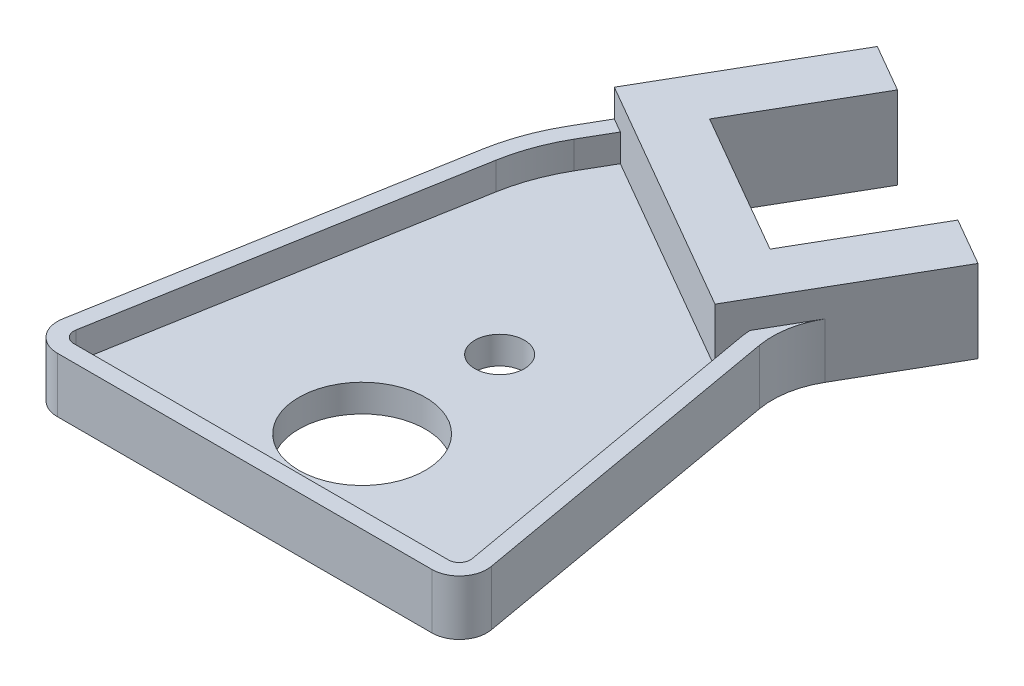
ISO-10303-21;
HEADER;
FILE_DESCRIPTION(('STEP AP214'),'2;1');
FILE_NAME('part.step','',(''),(''),'','','');
FILE_SCHEMA(('AUTOMOTIVE_DESIGN { 1 0 10303 214 1 1 1 1 }'));
ENDSEC;
DATA;
#1=APPLICATION_CONTEXT('core data for automotive mechanical design processes');
#2=APPLICATION_PROTOCOL_DEFINITION('international standard','automotive_design',2000,#1);
#3=PRODUCT_CONTEXT('',#1,'mechanical');
#4=PRODUCT('Part','Part','',(#3));
#5=PRODUCT_RELATED_PRODUCT_CATEGORY('part','',(#4));
#6=PRODUCT_DEFINITION_FORMATION('','',#4);
#7=PRODUCT_DEFINITION_CONTEXT('part definition',#1,'design');
#8=PRODUCT_DEFINITION('design','',#6,#7);
#9=PRODUCT_DEFINITION_SHAPE('','',#8);
#10=(LENGTH_UNIT() NAMED_UNIT(*) SI_UNIT(.MILLI.,.METRE.));
#11=(NAMED_UNIT(*) PLANE_ANGLE_UNIT() SI_UNIT($,.RADIAN.));
#12=(NAMED_UNIT(*) SI_UNIT($,.STERADIAN.) SOLID_ANGLE_UNIT());
#13=UNCERTAINTY_MEASURE_WITH_UNIT(LENGTH_MEASURE(1.E-05),#10,'distance_accuracy_value','');
#14=(GEOMETRIC_REPRESENTATION_CONTEXT(3) GLOBAL_UNCERTAINTY_ASSIGNED_CONTEXT((#13)) GLOBAL_UNIT_ASSIGNED_CONTEXT((#10,
#11,#12)) REPRESENTATION_CONTEXT('',''));
#15=CARTESIAN_POINT('',(0.,0.,0.));
#16=DIRECTION('',(0.,0.,1.));
#17=DIRECTION('',(1.,0.,0.));
#18=AXIS2_PLACEMENT_3D('',#15,#16,#17);
#19=CARTESIAN_POINT('',(5.58841015037912,10.,-64.6794103139903));
#20=DIRECTION('',(0.,-1.,0.));
#21=DIRECTION('',(0.,0.,-1.));
#22=AXIS2_PLACEMENT_3D('',#19,#20,#21);
#23=CYLINDRICAL_SURFACE('',#22,32.);
#24=CARTESIAN_POINT('',(5.58841015037912,5.,-64.6794103139903));
#25=DIRECTION('',(0.,1.,0.));
#26=DIRECTION('',(0.,0.,1.));
#27=AXIS2_PLACEMENT_3D('',#24,#25,#26);
#28=CIRCLE('',#27,32.);
#29=CARTESIAN_POINT('',(-22.1244027707229,5.,-80.6794103139904));
#30=VERTEX_POINT('',#29);
#31=CARTESIAN_POINT('',(-25.9254379460116,5.,-70.2361519993319));
#32=VERTEX_POINT('',#31);
#33=EDGE_CURVE('E290',#30,#32,#28,.T.);
#34=ORIENTED_EDGE('',*,*,#33,.F.);
#35=DIRECTION('',(0.,-1.,0.));
#36=VECTOR('',#35,1.);
#37=CARTESIAN_POINT('',(-22.1244027707229,10.,-80.6794103139904));
#38=LINE('',#37,#36);
#39=CARTESIAN_POINT('',(-22.1244027707229,10.,-80.6794103139904));
#40=VERTEX_POINT('',#39);
#41=EDGE_CURVE('E403',#40,#30,#38,.T.);
#42=ORIENTED_EDGE('',*,*,#41,.F.);
#43=CARTESIAN_POINT('',(5.58841015037912,10.,-64.6794103139903));
#44=DIRECTION('',(0.,1.,0.));
#45=DIRECTION('',(0.,0.,1.));
#46=AXIS2_PLACEMENT_3D('',#43,#44,#45);
#47=CIRCLE('',#46,32.);
#48=CARTESIAN_POINT('',(-25.9254379460116,10.,-70.2361519993319));
#49=VERTEX_POINT('',#48);
#50=EDGE_CURVE('E337',#49,#40,#47,.F.);
#51=ORIENTED_EDGE('',*,*,#50,.F.);
#52=DIRECTION('',(0.,-1.,0.));
#53=VECTOR('',#52,1.);
#54=CARTESIAN_POINT('',(-25.9254379460116,10.,-70.2361519993319));
#55=LINE('',#54,#53);
#56=EDGE_CURVE('E407',#49,#32,#55,.T.);
#57=ORIENTED_EDGE('',*,*,#56,.T.);
#58=EDGE_LOOP('',(#34,#42,#51,#57));
#59=FACE_BOUND('',#58,.T.);
#60=ADVANCED_FACE('F41',(#59),#23,.F.);
#61=CARTESIAN_POINT('',(41.9461329264872,10.,-67.6528334097137));
#62=DIRECTION('',(0.,-1.,0.));
#63=DIRECTION('',(0.,0.,-1.));
#64=AXIS2_PLACEMENT_3D('',#61,#62,#63);
#65=CYLINDRICAL_SURFACE('',#64,18.);
#66=DIRECTION('',(0.,-1.,0.));
#67=VECTOR('',#66,1.);
#68=CARTESIAN_POINT('',(23.9808146841875,10.,-66.5359894399066));
#69=LINE('',#68,#67);
#70=CARTESIAN_POINT('',(23.9808146841875,10.,-66.5359894399066));
#71=VERTEX_POINT('',#70);
#72=CARTESIAN_POINT('',(23.9808146841875,5.,-66.5359894399066));
#73=VERTEX_POINT('',#72);
#74=EDGE_CURVE('E11',#71,#73,#69,.T.);
#75=ORIENTED_EDGE('',*,*,#74,.T.);
#76=CARTESIAN_POINT('',(41.9461329264872,5.,-67.6528334097137));
#77=DIRECTION('',(0.,1.,0.));
#78=DIRECTION('',(0.,0.,1.));
#79=AXIS2_PLACEMENT_3D('',#76,#77,#78);
#80=CIRCLE('',#79,18.);
#81=CARTESIAN_POINT('',(24.2195933722675,5.,-64.527166211709));
#82=VERTEX_POINT('',#81);
#83=EDGE_CURVE('E64',#73,#82,#80,.T.);
#84=ORIENTED_EDGE('',*,*,#83,.T.);
#85=DIRECTION('',(0.,-1.,0.));
#86=VECTOR('',#85,1.);
#87=CARTESIAN_POINT('',(24.2195933722675,10.,-64.527166211709));
#88=LINE('',#87,#86);
#89=CARTESIAN_POINT('',(24.2195933722675,10.,-64.527166211709));
#90=VERTEX_POINT('',#89);
#91=EDGE_CURVE('E47',#90,#82,#88,.T.);
#92=ORIENTED_EDGE('',*,*,#91,.F.);
#93=CARTESIAN_POINT('',(41.9461329264872,10.,-67.6528334097137));
#94=DIRECTION('',(0.,1.,0.));
#95=DIRECTION('',(0.,0.,1.));
#96=AXIS2_PLACEMENT_3D('',#93,#94,#95);
#97=CIRCLE('',#96,18.);
#98=EDGE_CURVE('E317',#71,#90,#97,.T.);
#99=ORIENTED_EDGE('',*,*,#98,.F.);
#100=EDGE_LOOP('',(#75,#84,#92,#99));
#101=FACE_BOUND('',#100,.T.);
#102=ADVANCED_FACE('F43',(#101),#65,.T.);
#103=CARTESIAN_POINT('',(34.5240785893749,10.,-6.08752653940599));
#104=DIRECTION('',(-0.984807753012209,0.,0.173648177666924));
#105=DIRECTION('',(0.173648177666924,0.,0.984807753012209));
#106=AXIS2_PLACEMENT_3D('',#103,#104,#105);
#107=PLANE('',#106);
#108=DIRECTION('',(-0.173648177666924,0.,-0.984807753012209));
#109=VECTOR('',#108,1.);
#110=CARTESIAN_POINT('',(34.5240785893749,5.,-6.08752653940599));
#111=LINE('',#110,#109);
#112=CARTESIAN_POINT('',(34.6546011427616,5.,-5.34729635533385));
#113=VERTEX_POINT('',#112);
#114=EDGE_CURVE('E305',#113,#82,#111,.T.);
#115=ORIENTED_EDGE('',*,*,#114,.F.);
#116=DIRECTION('',(0.,-1.,0.));
#117=VECTOR('',#116,1.);
#118=CARTESIAN_POINT('',(34.6546011427616,10.,-5.34729635533385));
#119=LINE('',#118,#117);
#120=CARTESIAN_POINT('',(34.6546011427616,10.,-5.34729635533385));
#121=VERTEX_POINT('',#120);
#122=EDGE_CURVE('E420',#121,#113,#119,.T.);
#123=ORIENTED_EDGE('',*,*,#122,.F.);
#124=DIRECTION('',(-0.173648177666924,0.,-0.984807753012209));
#125=VECTOR('',#124,1.);
#126=CARTESIAN_POINT('',(34.5240785893749,10.,-6.08752653940599));
#127=LINE('',#126,#125);
#128=EDGE_CURVE('E325',#121,#90,#127,.T.);
#129=ORIENTED_EDGE('',*,*,#128,.T.);
#130=ORIENTED_EDGE('',*,*,#91,.T.);
#131=EDGE_LOOP('',(#115,#123,#129,#130));
#132=FACE_BOUND('',#131,.T.);
#133=ADVANCED_FACE('F425',(#132),#107,.T.);
#134=CARTESIAN_POINT('',(32.6849856367371,10.,-5.));
#135=DIRECTION('',(0.,-1.,0.));
#136=DIRECTION('',(0.,0.,-1.));
#137=AXIS2_PLACEMENT_3D('',#134,#135,#136);
#138=CYLINDRICAL_SURFACE('',#137,2.);
#139=CARTESIAN_POINT('',(32.6849856367371,5.,-5.));
#140=DIRECTION('',(0.,1.,0.));
#141=DIRECTION('',(0.,0.,1.));
#142=AXIS2_PLACEMENT_3D('',#139,#140,#141);
#143=CIRCLE('',#142,2.);
#144=CARTESIAN_POINT('',(32.6849856367371,5.,-3.));
#145=VERTEX_POINT('',#144);
#146=EDGE_CURVE('E298',#145,#113,#143,.T.);
#147=ORIENTED_EDGE('',*,*,#146,.F.);
#148=DIRECTION('',(0.,-1.,0.));
#149=VECTOR('',#148,1.);
#150=CARTESIAN_POINT('',(32.6849856367371,10.,-3.));
#151=LINE('',#150,#149);
#152=CARTESIAN_POINT('',(32.6849856367371,10.,-3.));
#153=VERTEX_POINT('',#152);
#154=EDGE_CURVE('E418',#153,#145,#151,.T.);
#155=ORIENTED_EDGE('',*,*,#154,.F.);
#156=CARTESIAN_POINT('',(32.6849856367371,10.,-5.));
#157=DIRECTION('',(0.,1.,0.));
#158=DIRECTION('',(0.,0.,1.));
#159=AXIS2_PLACEMENT_3D('',#156,#157,#158);
#160=CIRCLE('',#159,2.);
#161=EDGE_CURVE('E324',#153,#121,#160,.T.);
#162=ORIENTED_EDGE('',*,*,#161,.T.);
#163=ORIENTED_EDGE('',*,*,#122,.T.);
#164=EDGE_LOOP('',(#147,#155,#162,#163));
#165=FACE_BOUND('',#164,.T.);
#166=ADVANCED_FACE('F428',(#165),#138,.F.);
#167=CARTESIAN_POINT('',(0.,10.,-3.));
#168=DIRECTION('',(0.,0.,-1.));
#169=DIRECTION('',(-1.,0.,0.));
#170=AXIS2_PLACEMENT_3D('',#167,#168,#169);
#171=PLANE('',#170);
#172=DIRECTION('',(1.,0.,0.));
#173=VECTOR('',#172,1.);
#174=CARTESIAN_POINT('',(0.,5.,-3.));
#175=LINE('',#174,#173);
#176=CARTESIAN_POINT('',(-35.3974784373208,5.,-3.));
#177=VERTEX_POINT('',#176);
#178=EDGE_CURVE('E296',#177,#145,#175,.T.);
#179=ORIENTED_EDGE('',*,*,#178,.F.);
#180=DIRECTION('',(0.,-1.,0.));
#181=VECTOR('',#180,1.);
#182=CARTESIAN_POINT('',(-35.3974784373208,10.,-3.));
#183=LINE('',#182,#181);
#184=CARTESIAN_POINT('',(-35.3974784373208,10.,-3.));
#185=VERTEX_POINT('',#184);
#186=EDGE_CURVE('E413',#185,#177,#183,.T.);
#187=ORIENTED_EDGE('',*,*,#186,.F.);
#188=DIRECTION('',(1.,0.,0.));
#189=VECTOR('',#188,1.);
#190=CARTESIAN_POINT('',(0.,10.,-3.));
#191=LINE('',#190,#189);
#192=EDGE_CURVE('E327',#185,#153,#191,.T.);
#193=ORIENTED_EDGE('',*,*,#192,.T.);
#194=ORIENTED_EDGE('',*,*,#154,.T.);
#195=EDGE_LOOP('',(#179,#187,#193,#194));
#196=FACE_BOUND('',#195,.T.);
#197=ADVANCED_FACE('F431',(#196),#171,.T.);
#198=CARTESIAN_POINT('',(-35.3974784373208,10.,-5.));
#199=DIRECTION('',(0.,-1.,0.));
#200=DIRECTION('',(0.,0.,-1.));
#201=AXIS2_PLACEMENT_3D('',#198,#199,#200);
#202=CYLINDRICAL_SURFACE('',#201,2.);
#203=CARTESIAN_POINT('',(-35.3974784373208,5.,-5.));
#204=DIRECTION('',(0.,1.,0.));
#205=DIRECTION('',(0.,0.,1.));
#206=AXIS2_PLACEMENT_3D('',#203,#204,#205);
#207=CIRCLE('',#206,2.);
#208=CARTESIAN_POINT('',(-37.3670939433452,5.,-5.34729635533386));
#209=VERTEX_POINT('',#208);
#210=EDGE_CURVE('E291',#209,#177,#207,.T.);
#211=ORIENTED_EDGE('',*,*,#210,.F.);
#212=DIRECTION('',(0.,-1.,0.));
#213=VECTOR('',#212,1.);
#214=CARTESIAN_POINT('',(-37.3670939433452,10.,-5.34729635533386));
#215=LINE('',#214,#213);
#216=CARTESIAN_POINT('',(-37.3670939433452,10.,-5.34729635533386));
#217=VERTEX_POINT('',#216);
#218=EDGE_CURVE('E410',#217,#209,#215,.T.);
#219=ORIENTED_EDGE('',*,*,#218,.F.);
#220=CARTESIAN_POINT('',(-35.3974784373208,10.,-5.));
#221=DIRECTION('',(0.,1.,0.));
#222=DIRECTION('',(0.,0.,1.));
#223=AXIS2_PLACEMENT_3D('',#220,#221,#222);
#224=CIRCLE('',#223,2.);
#225=EDGE_CURVE('E332',#217,#185,#224,.T.);
#226=ORIENTED_EDGE('',*,*,#225,.T.);
#227=ORIENTED_EDGE('',*,*,#186,.T.);
#228=EDGE_LOOP('',(#211,#219,#226,#227));
#229=FACE_BOUND('',#228,.T.);
#230=ADVANCED_FACE('F438',(#229),#202,.F.);
#231=CARTESIAN_POINT('',(-37.1547797239883,10.,-6.55139012761897));
#232=DIRECTION('',(0.984807753012208,0.,0.173648177666931));
#233=DIRECTION('',(0.173648177666931,0.,-0.984807753012208));
#234=AXIS2_PLACEMENT_3D('',#231,#232,#233);
#235=PLANE('',#234);
#236=DIRECTION('',(-0.173648177666931,0.,0.984807753012208));
#237=VECTOR('',#236,1.);
#238=CARTESIAN_POINT('',(-37.1547797239883,5.,-6.55139012761897));
#239=LINE('',#238,#237);
#240=EDGE_CURVE('E289',#32,#209,#239,.T.);
#241=ORIENTED_EDGE('',*,*,#240,.F.);
#242=ORIENTED_EDGE('',*,*,#56,.F.);
#243=DIRECTION('',(-0.173648177666931,0.,0.984807753012208));
#244=VECTOR('',#243,1.);
#245=CARTESIAN_POINT('',(-37.1547797239883,10.,-6.55139012761897));
#246=LINE('',#245,#244);
#247=EDGE_CURVE('E331',#49,#217,#246,.T.);
#248=ORIENTED_EDGE('',*,*,#247,.T.);
#249=ORIENTED_EDGE('',*,*,#218,.T.);
#250=EDGE_LOOP('',(#241,#242,#248,#249));
#251=FACE_BOUND('',#250,.T.);
#252=ADVANCED_FACE('F442',(#251),#235,.T.);
#253=CARTESIAN_POINT('',(-51.5285115251741,10.,-29.75));
#254=DIRECTION('',(0.866025403784439,0.,0.5));
#255=DIRECTION('',(0.5,0.,-0.866025403784439));
#256=AXIS2_PLACEMENT_3D('',#253,#254,#255);
#257=PLANE('',#256);
#258=DIRECTION('',(-0.500000000000001,0.,0.866025403784438));
#259=VECTOR('',#258,1.);
#260=CARTESIAN_POINT('',(-51.5285115251741,5.,-29.7500000000001));
#261=LINE('',#260,#259);
#262=CARTESIAN_POINT('',(-19.0525588832577,5.,-86.));
#263=VERTEX_POINT('',#262);
#264=EDGE_CURVE('E57',#263,#30,#261,.T.);
#265=ORIENTED_EDGE('',*,*,#264,.F.);
#266=DIRECTION('',(0.,-1.,0.));
#267=VECTOR('',#266,1.);
#268=CARTESIAN_POINT('',(-19.0525588832577,10.,-86.));
#269=LINE('',#268,#267);
#270=CARTESIAN_POINT('',(-19.0525588832577,10.,-86.));
#271=VERTEX_POINT('',#270);
#272=EDGE_CURVE('E405',#271,#263,#269,.T.);
#273=ORIENTED_EDGE('',*,*,#272,.F.);
#274=DIRECTION('',(-0.5,0.,0.866025403784439));
#275=VECTOR('',#274,1.);
#276=CARTESIAN_POINT('',(-51.5285115251741,10.,-29.75));
#277=LINE('',#276,#275);
#278=EDGE_CURVE('E338',#271,#40,#277,.T.);
#279=ORIENTED_EDGE('',*,*,#278,.T.);
#280=ORIENTED_EDGE('',*,*,#41,.T.);
#281=EDGE_LOOP('',(#265,#273,#279,#280));
#282=FACE_BOUND('',#281,.T.);
#283=ADVANCED_FACE('F503',(#282),#257,.T.);
#284=CARTESIAN_POINT('',(-54.1265877365274,10.,-31.25));
#285=DIRECTION('',(0.866025403784439,0.,0.5));
#286=DIRECTION('',(0.5,0.,-0.866025403784439));
#287=AXIS2_PLACEMENT_3D('',#284,#285,#286);
#288=PLANE('',#287);
#289=DIRECTION('',(-0.5,0.,0.866025403784439));
#290=VECTOR('',#289,1.);
#291=CARTESIAN_POINT('',(-54.1265877365274,0.,-31.25));
#292=LINE('',#291,#290);
#293=CARTESIAN_POINT('',(-4.15063509461097,0.,-117.810889132455));
#294=VERTEX_POINT('',#293);
#295=CARTESIAN_POINT('',(-24.7224789820762,0.,-82.1794103139904));
#296=VERTEX_POINT('',#295);
#297=EDGE_CURVE('E313',#294,#296,#292,.T.);
#298=ORIENTED_EDGE('',*,*,#297,.T.);
#299=DIRECTION('',(0.,-1.,0.));
#300=VECTOR('',#299,1.);
#301=CARTESIAN_POINT('',(-24.7224789820762,10.,-82.1794103139904));
#302=LINE('',#301,#300);
#303=CARTESIAN_POINT('',(-24.7224789820762,10.,-82.1794103139904));
#304=VERTEX_POINT('',#303);
#305=EDGE_CURVE('E399',#304,#296,#302,.T.);
#306=ORIENTED_EDGE('',*,*,#305,.F.);
#307=DIRECTION('',(-0.5,0.,0.866025403784439));
#308=VECTOR('',#307,1.);
#309=CARTESIAN_POINT('',(-54.1265877365274,10.,-31.25));
#310=LINE('',#309,#308);
#311=CARTESIAN_POINT('',(-21.650635094611,10.,-87.5));
#312=VERTEX_POINT('',#311);
#313=EDGE_CURVE('E344',#312,#304,#310,.T.);
#314=ORIENTED_EDGE('',*,*,#313,.F.);
#315=DIRECTION('',(0.,-1.,0.));
#316=VECTOR('',#315,1.);
#317=CARTESIAN_POINT('',(-21.650635094611,15.,-87.5));
#318=LINE('',#317,#316);
#319=CARTESIAN_POINT('',(-21.650635094611,15.,-87.5));
#320=VERTEX_POINT('',#319);
#321=EDGE_CURVE('E273',#320,#312,#318,.T.);
#322=ORIENTED_EDGE('',*,*,#321,.F.);
#323=DIRECTION('',(-0.5,0.,0.866025403784439));
#324=VECTOR('',#323,1.);
#325=CARTESIAN_POINT('',(-54.1265877365274,15.,-31.25));
#326=LINE('',#325,#324);
#327=CARTESIAN_POINT('',(-4.15063509461097,15.,-117.810889132455));
#328=VERTEX_POINT('',#327);
#329=EDGE_CURVE('E232',#328,#320,#326,.T.);
#330=ORIENTED_EDGE('',*,*,#329,.F.);
#331=DIRECTION('',(0.,-1.,0.));
#332=VECTOR('',#331,1.);
#333=CARTESIAN_POINT('',(-4.15063509461097,15.,-117.810889132455));
#334=LINE('',#333,#332);
#335=EDGE_CURVE('E219',#328,#294,#334,.T.);
#336=ORIENTED_EDGE('',*,*,#335,.T.);
#337=EDGE_LOOP('',(#298,#306,#314,#322,#330,#336));
#338=FACE_BOUND('',#337,.T.);
#339=ADVANCED_FACE('F452',(#338),#288,.F.);
#340=CARTESIAN_POINT('',(5.58841015037912,10.,-64.6794103139903));
#341=DIRECTION('',(0.,-1.,0.));
#342=DIRECTION('',(0.,0.,-1.));
#343=AXIS2_PLACEMENT_3D('',#340,#341,#342);
#344=CYLINDRICAL_SURFACE('',#343,35.);
#345=CARTESIAN_POINT('',(5.58841015037912,0.,-64.6794103139903));
#346=DIRECTION('',(0.,1.,0.));
#347=DIRECTION('',(0.,0.,1.));
#348=AXIS2_PLACEMENT_3D('',#345,#346,#347);
#349=CIRCLE('',#348,35.);
#350=CARTESIAN_POINT('',(-28.8798612050482,0.,-70.7570965323327));
#351=VERTEX_POINT('',#350);
#352=EDGE_CURVE('E368',#351,#296,#349,.F.);
#353=ORIENTED_EDGE('',*,*,#352,.F.);
#354=DIRECTION('',(0.,-1.,0.));
#355=VECTOR('',#354,1.);
#356=CARTESIAN_POINT('',(-28.8798612050482,10.,-70.7570965323327));
#357=LINE('',#356,#355);
#358=CARTESIAN_POINT('',(-28.8798612050482,10.,-70.7570965323327));
#359=VERTEX_POINT('',#358);
#360=EDGE_CURVE('E398',#359,#351,#357,.T.);
#361=ORIENTED_EDGE('',*,*,#360,.F.);
#362=CARTESIAN_POINT('',(5.58841015037912,10.,-64.6794103139903));
#363=DIRECTION('',(0.,1.,0.));
#364=DIRECTION('',(0.,0.,1.));
#365=AXIS2_PLACEMENT_3D('',#362,#363,#364);
#366=CIRCLE('',#365,35.);
#367=EDGE_CURVE('E350',#359,#304,#366,.F.);
#368=ORIENTED_EDGE('',*,*,#367,.T.);
#369=ORIENTED_EDGE('',*,*,#305,.T.);
#370=EDGE_LOOP('',(#353,#361,#368,#369));
#371=FACE_BOUND('',#370,.T.);
#372=ADVANCED_FACE('F461',(#371),#344,.T.);
#373=CARTESIAN_POINT('',(-40.1092029830249,10.,-7.07233466061976));
#374=DIRECTION('',(0.984807753012208,0.,0.173648177666931));
#375=DIRECTION('',(0.173648177666931,0.,-0.984807753012208));
#376=AXIS2_PLACEMENT_3D('',#373,#374,#375);
#377=PLANE('',#376);
#378=DIRECTION('',(-0.173648177666931,0.,0.984807753012208));
#379=VECTOR('',#378,1.);
#380=CARTESIAN_POINT('',(-40.1092029830249,0.,-7.07233466061976));
#381=LINE('',#380,#379);
#382=CARTESIAN_POINT('',(-40.3215172023818,0.,-5.86824088833466));
#383=VERTEX_POINT('',#382);
#384=EDGE_CURVE('E369',#351,#383,#381,.T.);
#385=ORIENTED_EDGE('',*,*,#384,.T.);
#386=DIRECTION('',(0.,-1.,0.));
#387=VECTOR('',#386,1.);
#388=CARTESIAN_POINT('',(-40.3215172023818,10.,-5.86824088833466));
#389=LINE('',#388,#387);
#390=CARTESIAN_POINT('',(-40.3215172023818,10.,-5.86824088833466));
#391=VERTEX_POINT('',#390);
#392=EDGE_CURVE('E395',#391,#383,#389,.T.);
#393=ORIENTED_EDGE('',*,*,#392,.F.);
#394=DIRECTION('',(-0.173648177666931,0.,0.984807753012208));
#395=VECTOR('',#394,1.);
#396=CARTESIAN_POINT('',(-40.1092029830249,10.,-7.07233466061976));
#397=LINE('',#396,#395);
#398=EDGE_CURVE('E348',#359,#391,#397,.T.);
#399=ORIENTED_EDGE('',*,*,#398,.F.);
#400=ORIENTED_EDGE('',*,*,#360,.T.);
#401=EDGE_LOOP('',(#385,#393,#399,#400));
#402=FACE_BOUND('',#401,.T.);
#403=ADVANCED_FACE('F463',(#402),#377,.F.);
#404=CARTESIAN_POINT('',(-35.3974784373208,10.,-5.));
#405=DIRECTION('',(0.,-1.,0.));
#406=DIRECTION('',(0.,0.,-1.));
#407=AXIS2_PLACEMENT_3D('',#404,#405,#406);
#408=CYLINDRICAL_SURFACE('',#407,5.);
#409=CARTESIAN_POINT('',(-35.3974784373208,0.,-5.));
#410=DIRECTION('',(0.,1.,0.));
#411=DIRECTION('',(0.,0.,1.));
#412=AXIS2_PLACEMENT_3D('',#409,#410,#411);
#413=CIRCLE('',#412,5.);
#414=CARTESIAN_POINT('',(-35.3974784373208,0.,0.));
#415=VERTEX_POINT('',#414);
#416=EDGE_CURVE('E371',#383,#415,#413,.T.);
#417=ORIENTED_EDGE('',*,*,#416,.T.);
#418=DIRECTION('',(0.,-1.,0.));
#419=VECTOR('',#418,1.);
#420=CARTESIAN_POINT('',(-35.3974784373208,10.,0.));
#421=LINE('',#420,#419);
#422=CARTESIAN_POINT('',(-35.3974784373208,10.,0.));
#423=VERTEX_POINT('',#422);
#424=EDGE_CURVE('E392',#423,#415,#421,.T.);
#425=ORIENTED_EDGE('',*,*,#424,.F.);
#426=CARTESIAN_POINT('',(-35.3974784373208,10.,-5.));
#427=DIRECTION('',(0.,1.,0.));
#428=DIRECTION('',(0.,0.,1.));
#429=AXIS2_PLACEMENT_3D('',#426,#427,#428);
#430=CIRCLE('',#429,5.);
#431=EDGE_CURVE('E352',#391,#423,#430,.T.);
#432=ORIENTED_EDGE('',*,*,#431,.F.);
#433=ORIENTED_EDGE('',*,*,#392,.T.);
#434=EDGE_LOOP('',(#417,#425,#432,#433));
#435=FACE_BOUND('',#434,.T.);
#436=ADVANCED_FACE('F467',(#435),#408,.T.);
#437=CARTESIAN_POINT('',(0.,10.,0.));
#438=DIRECTION('',(0.,0.,-1.));
#439=DIRECTION('',(-1.,0.,0.));
#440=AXIS2_PLACEMENT_3D('',#437,#438,#439);
#441=PLANE('',#440);
#442=DIRECTION('',(1.,0.,0.));
#443=VECTOR('',#442,1.);
#444=CARTESIAN_POINT('',(0.,0.,0.));
#445=LINE('',#444,#443);
#446=CARTESIAN_POINT('',(32.6849856367371,0.,0.));
#447=VERTEX_POINT('',#446);
#448=EDGE_CURVE('E373',#415,#447,#445,.T.);
#449=ORIENTED_EDGE('',*,*,#448,.T.);
#450=DIRECTION('',(0.,-1.,0.));
#451=VECTOR('',#450,1.);
#452=CARTESIAN_POINT('',(32.6849856367371,10.,0.));
#453=LINE('',#452,#451);
#454=CARTESIAN_POINT('',(32.6849856367371,10.,0.));
#455=VERTEX_POINT('',#454);
#456=EDGE_CURVE('E386',#455,#447,#453,.T.);
#457=ORIENTED_EDGE('',*,*,#456,.F.);
#458=DIRECTION('',(1.,0.,0.));
#459=VECTOR('',#458,1.);
#460=CARTESIAN_POINT('',(0.,10.,0.));
#461=LINE('',#460,#459);
#462=EDGE_CURVE('E353',#423,#455,#461,.T.);
#463=ORIENTED_EDGE('',*,*,#462,.F.);
#464=ORIENTED_EDGE('',*,*,#424,.T.);
#465=EDGE_LOOP('',(#449,#457,#463,#464));
#466=FACE_BOUND('',#465,.T.);
#467=ADVANCED_FACE('F474',(#466),#441,.F.);
#468=CARTESIAN_POINT('',(32.6849856367371,10.,-5.));
#469=DIRECTION('',(0.,-1.,0.));
#470=DIRECTION('',(0.,0.,-1.));
#471=AXIS2_PLACEMENT_3D('',#468,#469,#470);
#472=CYLINDRICAL_SURFACE('',#471,5.);
#473=CARTESIAN_POINT('',(32.6849856367371,0.,-5.));
#474=DIRECTION('',(0.,1.,0.));
#475=DIRECTION('',(0.,0.,1.));
#476=AXIS2_PLACEMENT_3D('',#473,#474,#475);
#477=CIRCLE('',#476,5.);
#478=CARTESIAN_POINT('',(37.6090244017982,0.,-5.86824088833462));
#479=VERTEX_POINT('',#478);
#480=EDGE_CURVE('E374',#447,#479,#477,.T.);
#481=ORIENTED_EDGE('',*,*,#480,.T.);
#482=DIRECTION('',(0.,-1.,0.));
#483=VECTOR('',#482,1.);
#484=CARTESIAN_POINT('',(37.6090244017982,10.,-5.86824088833462));
#485=LINE('',#484,#483);
#486=CARTESIAN_POINT('',(37.6090244017982,10.,-5.86824088833462));
#487=VERTEX_POINT('',#486);
#488=EDGE_CURVE('E387',#487,#479,#485,.T.);
#489=ORIENTED_EDGE('',*,*,#488,.F.);
#490=CARTESIAN_POINT('',(32.6849856367371,10.,-5.));
#491=DIRECTION('',(0.,1.,0.));
#492=DIRECTION('',(0.,0.,1.));
#493=AXIS2_PLACEMENT_3D('',#490,#491,#492);
#494=CIRCLE('',#493,5.);
#495=EDGE_CURVE('E356',#455,#487,#494,.T.);
#496=ORIENTED_EDGE('',*,*,#495,.F.);
#497=ORIENTED_EDGE('',*,*,#456,.T.);
#498=EDGE_LOOP('',(#481,#489,#496,#497));
#499=FACE_BOUND('',#498,.T.);
#500=ADVANCED_FACE('F479',(#499),#472,.T.);
#501=CARTESIAN_POINT('',(37.4785018484115,10.,-6.60847107240677));
#502=DIRECTION('',(-0.984807753012209,0.,0.173648177666924));
#503=DIRECTION('',(0.173648177666924,0.,0.984807753012209));
#504=AXIS2_PLACEMENT_3D('',#501,#502,#503);
#505=PLANE('',#504);
#506=DIRECTION('',(-0.173648177666924,0.,-0.984807753012209));
#507=VECTOR('',#506,1.);
#508=CARTESIAN_POINT('',(37.4785018484115,0.,-6.60847107240677));
#509=LINE('',#508,#507);
#510=CARTESIAN_POINT('',(27.1740166313041,0.,-65.0481107447097));
#511=VERTEX_POINT('',#510);
#512=EDGE_CURVE('E380',#479,#511,#509,.T.);
#513=ORIENTED_EDGE('',*,*,#512,.T.);
#514=DIRECTION('',(0.,-1.,0.));
#515=VECTOR('',#514,1.);
#516=CARTESIAN_POINT('',(27.1740166313041,10.,-65.0481107447097));
#517=LINE('',#516,#515);
#518=CARTESIAN_POINT('',(27.1740166313041,10.,-65.0481107447097));
#519=VERTEX_POINT('',#518);
#520=EDGE_CURVE('E383',#519,#511,#517,.T.);
#521=ORIENTED_EDGE('',*,*,#520,.F.);
#522=DIRECTION('',(-0.173648177666924,0.,-0.984807753012209));
#523=VECTOR('',#522,1.);
#524=CARTESIAN_POINT('',(37.4785018484115,10.,-6.60847107240677));
#525=LINE('',#524,#523);
#526=EDGE_CURVE('E358',#487,#519,#525,.T.);
#527=ORIENTED_EDGE('',*,*,#526,.F.);
#528=ORIENTED_EDGE('',*,*,#488,.T.);
#529=EDGE_LOOP('',(#513,#521,#527,#528));
#530=FACE_BOUND('',#529,.T.);
#531=ADVANCED_FACE('F482',(#530),#505,.F.);
#532=CARTESIAN_POINT('',(41.9461329264872,10.,-67.6528334097137));
#533=DIRECTION('',(0.,-1.,0.));
#534=DIRECTION('',(0.,0.,-1.));
#535=AXIS2_PLACEMENT_3D('',#532,#533,#534);
#536=CYLINDRICAL_SURFACE('',#535,15.);
#537=CARTESIAN_POINT('',(41.9461329264872,0.,-67.6528334097137));
#538=DIRECTION('',(0.,1.,0.));
#539=DIRECTION('',(0.,0.,1.));
#540=AXIS2_PLACEMENT_3D('',#537,#538,#539);
#541=CIRCLE('',#540,15.);
#542=CARTESIAN_POINT('',(28.9557518697206,0.,-75.1528334097136));
#543=VERTEX_POINT('',#542);
#544=EDGE_CURVE('E319',#543,#511,#541,.T.);
#545=ORIENTED_EDGE('',*,*,#544,.F.);
#546=DIRECTION('',(0.,-1.,0.));
#547=VECTOR('',#546,1.);
#548=CARTESIAN_POINT('',(28.9557518697206,10.,-75.1528334097136));
#549=LINE('',#548,#547);
#550=CARTESIAN_POINT('',(28.9557518697206,10.,-75.1528334097136));
#551=VERTEX_POINT('',#550);
#552=EDGE_CURVE('E361',#551,#543,#549,.T.);
#553=ORIENTED_EDGE('',*,*,#552,.F.);
#554=CARTESIAN_POINT('',(41.9461329264872,10.,-67.6528334097137));
#555=DIRECTION('',(0.,1.,0.));
#556=DIRECTION('',(0.,0.,1.));
#557=AXIS2_PLACEMENT_3D('',#554,#555,#556);
#558=CIRCLE('',#557,15.);
#559=EDGE_CURVE('E359',#551,#519,#558,.T.);
#560=ORIENTED_EDGE('',*,*,#559,.T.);
#561=ORIENTED_EDGE('',*,*,#520,.T.);
#562=EDGE_LOOP('',(#545,#553,#560,#561));
#563=FACE_BOUND('',#562,.T.);
#564=ADVANCED_FACE('F657',(#563),#536,.F.);
#565=CARTESIAN_POINT('',(0.,10.,0.));
#566=DIRECTION('',(0.,1.,0.));
#567=DIRECTION('',(0.,0.,1.));
#568=AXIS2_PLACEMENT_3D('',#565,#566,#567);
#569=PLANE('',#568);
#570=DIRECTION('',(0.5,0.,-0.866025403784439));
#571=VECTOR('',#570,1.);
#572=CARTESIAN_POINT('',(-10.8253175473055,10.,-6.25));
#573=LINE('',#572,#571);
#574=EDGE_CURVE('E316',#71,#551,#573,.T.);
#575=ORIENTED_EDGE('',*,*,#574,.F.);
#576=ORIENTED_EDGE('',*,*,#98,.T.);
#577=ORIENTED_EDGE('',*,*,#128,.F.);
#578=ORIENTED_EDGE('',*,*,#161,.F.);
#579=ORIENTED_EDGE('',*,*,#192,.F.);
#580=ORIENTED_EDGE('',*,*,#225,.F.);
#581=ORIENTED_EDGE('',*,*,#247,.F.);
#582=ORIENTED_EDGE('',*,*,#50,.T.);
#583=ORIENTED_EDGE('',*,*,#278,.F.);
#584=DIRECTION('',(0.866025403784439,0.,0.5));
#585=VECTOR('',#584,1.);
#586=CARTESIAN_POINT('',(32.4759526419164,10.,-56.25));
#587=LINE('',#586,#585);
#588=EDGE_CURVE('E345',#312,#271,#587,.T.);
#589=ORIENTED_EDGE('',*,*,#588,.F.);
#590=ORIENTED_EDGE('',*,*,#313,.T.);
#591=ORIENTED_EDGE('',*,*,#367,.F.);
#592=ORIENTED_EDGE('',*,*,#398,.T.);
#593=ORIENTED_EDGE('',*,*,#431,.T.);
#594=ORIENTED_EDGE('',*,*,#462,.T.);
#595=ORIENTED_EDGE('',*,*,#495,.T.);
#596=ORIENTED_EDGE('',*,*,#526,.T.);
#597=ORIENTED_EDGE('',*,*,#559,.F.);
#598=EDGE_LOOP('',(#575,#576,#577,#578,#579,#580,#581,#582,#583,#589,#590,#591,#592,#593,#594,
#595,#596,#597));
#599=FACE_BOUND('',#598,.T.);
#600=ADVANCED_FACE('F436',(#599),#569,.T.);
#601=CARTESIAN_POINT('',(0.,0.,0.));
#602=DIRECTION('',(0.,1.,0.));
#603=DIRECTION('',(0.,0.,1.));
#604=AXIS2_PLACEMENT_3D('',#601,#602,#603);
#605=PLANE('',#604);
#606=DIRECTION('',(0.5,0.,-0.866025403784439));
#607=VECTOR('',#606,1.);
#608=CARTESIAN_POINT('',(-10.8253175473055,0.,-6.25));
#609=LINE('',#608,#607);
#610=CARTESIAN_POINT('',(39.1506350946109,0.,-92.8108891324554));
#611=VERTEX_POINT('',#610);
#612=EDGE_CURVE('E251',#543,#611,#609,.T.);
#613=ORIENTED_EDGE('',*,*,#612,.F.);
#614=ORIENTED_EDGE('',*,*,#544,.T.);
#615=ORIENTED_EDGE('',*,*,#512,.F.);
#616=ORIENTED_EDGE('',*,*,#480,.F.);
#617=ORIENTED_EDGE('',*,*,#448,.F.);
#618=ORIENTED_EDGE('',*,*,#416,.F.);
#619=ORIENTED_EDGE('',*,*,#384,.F.);
#620=ORIENTED_EDGE('',*,*,#352,.T.);
#621=ORIENTED_EDGE('',*,*,#297,.F.);
#622=DIRECTION('',(0.866025403784438,0.,0.5));
#623=VECTOR('',#622,1.);
#624=CARTESIAN_POINT('',(49.9759526419165,0.,-86.5608891324553));
#625=LINE('',#624,#623);
#626=CARTESIAN_POINT('',(4.50961894323341,0.,-112.810889132455));
#627=VERTEX_POINT('',#626);
#628=EDGE_CURVE('E253',#294,#627,#625,.T.);
#629=ORIENTED_EDGE('',*,*,#628,.T.);
#630=DIRECTION('',(-0.5,0.,0.866025403784439));
#631=VECTOR('',#630,1.);
#632=CARTESIAN_POINT('',(-45.466333698683,0.,-26.2499999999999));
#633=LINE('',#632,#631);
#634=CARTESIAN_POINT('',(-7.99038105676658,0.,-91.1602540378444));
#635=VERTEX_POINT('',#634);
#636=EDGE_CURVE('E212',#627,#635,#633,.T.);
#637=ORIENTED_EDGE('',*,*,#636,.T.);
#638=DIRECTION('',(0.866025403784439,0.,0.5));
#639=VECTOR('',#638,1.);
#640=CARTESIAN_POINT('',(37.4759526419164,0.,-64.9102540378444));
#641=LINE('',#640,#639);
#642=CARTESIAN_POINT('',(17.9903810567666,0.,-76.1602540378444));
#643=VERTEX_POINT('',#642);
#644=EDGE_CURVE('E228',#635,#643,#641,.T.);
#645=ORIENTED_EDGE('',*,*,#644,.T.);
#646=DIRECTION('',(0.5,0.,-0.866025403784439));
#647=VECTOR('',#646,1.);
#648=CARTESIAN_POINT('',(-19.4855715851499,0.,-11.25));
#649=LINE('',#648,#647);
#650=CARTESIAN_POINT('',(30.4903810567666,0.,-97.8108891324553));
#651=VERTEX_POINT('',#650);
#652=EDGE_CURVE('E256',#643,#651,#649,.T.);
#653=ORIENTED_EDGE('',*,*,#652,.T.);
#654=DIRECTION('',(0.866025403784439,0.,0.5));
#655=VECTOR('',#654,1.);
#656=CARTESIAN_POINT('',(49.9759526419164,0.,-86.5608891324554));
#657=LINE('',#656,#655);
#658=EDGE_CURVE('E254',#651,#611,#657,.T.);
#659=ORIENTED_EDGE('',*,*,#658,.T.);
#660=EDGE_LOOP('',(#613,#614,#615,#616,#617,#618,#619,#620,#621,#629,#637,#645,#653,#659));
#661=FACE_BOUND('',#660,.T.);
#662=CARTESIAN_POINT('',(0.,0.,-45.));
#663=DIRECTION('',(0.,1.,0.));
#664=DIRECTION('',(0.,0.,1.));
#665=AXIS2_PLACEMENT_3D('',#662,#663,#664);
#666=CIRCLE('',#665,4.5);
#667=CARTESIAN_POINT('',(0.,0.,-40.5));
#668=VERTEX_POINT('',#667);
#669=EDGE_CURVE('E218',#668,#668,#666,.T.);
#670=ORIENTED_EDGE('',*,*,#669,.T.);
#671=EDGE_LOOP('',(#670));
#672=FACE_BOUND('',#671,.T.);
#673=CARTESIAN_POINT('',(0.,0.,-20.));
#674=DIRECTION('',(0.,1.,0.));
#675=DIRECTION('',(0.,0.,1.));
#676=AXIS2_PLACEMENT_3D('',#673,#674,#675);
#677=CIRCLE('',#676,11.5);
#678=CARTESIAN_POINT('',(0.,0.,-8.5));
#679=VERTEX_POINT('',#678);
#680=EDGE_CURVE('E278',#679,#679,#677,.T.);
#681=ORIENTED_EDGE('',*,*,#680,.T.);
#682=EDGE_LOOP('',(#681));
#683=FACE_BOUND('',#682,.T.);
#684=ADVANCED_FACE('F541',(#661,#672,#683),#605,.F.);
#685=CARTESIAN_POINT('',(0.,5.,-45.));
#686=DIRECTION('',(0.,-1.,0.));
#687=DIRECTION('',(0.,0.,-1.));
#688=AXIS2_PLACEMENT_3D('',#685,#686,#687);
#689=CYLINDRICAL_SURFACE('',#688,4.5);
#690=CARTESIAN_POINT('',(0.,5.,-45.));
#691=DIRECTION('',(0.,1.,0.));
#692=DIRECTION('',(0.,0.,1.));
#693=AXIS2_PLACEMENT_3D('',#690,#691,#692);
#694=CIRCLE('',#693,4.5);
#695=CARTESIAN_POINT('',(0.,5.,-40.5));
#696=VERTEX_POINT('',#695);
#697=EDGE_CURVE('E304',#696,#696,#694,.T.);
#698=ORIENTED_EDGE('',*,*,#697,.T.);
#699=EDGE_LOOP('',(#698));
#700=FACE_BOUND('',#699,.T.);
#701=ORIENTED_EDGE('',*,*,#669,.F.);
#702=EDGE_LOOP('',(#701));
#703=FACE_BOUND('',#702,.T.);
#704=ADVANCED_FACE('F540',(#700,#703),#689,.F.);
#705=CARTESIAN_POINT('',(0.,5.,-20.));
#706=DIRECTION('',(0.,-1.,0.));
#707=DIRECTION('',(0.,0.,-1.));
#708=AXIS2_PLACEMENT_3D('',#705,#706,#707);
#709=CYLINDRICAL_SURFACE('',#708,11.5);
#710=CARTESIAN_POINT('',(0.,5.,-20.));
#711=DIRECTION('',(0.,1.,0.));
#712=DIRECTION('',(0.,0.,1.));
#713=AXIS2_PLACEMENT_3D('',#710,#711,#712);
#714=CIRCLE('',#713,11.5);
#715=CARTESIAN_POINT('',(0.,5.,-8.5));
#716=VERTEX_POINT('',#715);
#717=EDGE_CURVE('E306',#716,#716,#714,.T.);
#718=ORIENTED_EDGE('',*,*,#717,.T.);
#719=EDGE_LOOP('',(#718));
#720=FACE_BOUND('',#719,.T.);
#721=ORIENTED_EDGE('',*,*,#680,.F.);
#722=EDGE_LOOP('',(#721));
#723=FACE_BOUND('',#722,.T.);
#724=ADVANCED_FACE('F539',(#720,#723),#709,.F.);
#725=CARTESIAN_POINT('',(0.,5.,0.));
#726=DIRECTION('',(0.,1.,0.));
#727=DIRECTION('',(0.,0.,1.));
#728=AXIS2_PLACEMENT_3D('',#725,#726,#727);
#729=PLANE('',#728);
#730=ORIENTED_EDGE('',*,*,#83,.F.);
#731=DIRECTION('',(0.5,0.,-0.866025403784439));
#732=VECTOR('',#731,1.);
#733=CARTESIAN_POINT('',(-10.8253175473055,5.,-6.25));
#734=LINE('',#733,#732);
#735=CARTESIAN_POINT('',(21.6506350946109,5.,-62.5));
#736=VERTEX_POINT('',#735);
#737=EDGE_CURVE('E276',#736,#73,#734,.T.);
#738=ORIENTED_EDGE('',*,*,#737,.F.);
#739=DIRECTION('',(0.866025403784439,0.,0.5));
#740=VECTOR('',#739,1.);
#741=CARTESIAN_POINT('',(32.4759526419164,5.,-56.25));
#742=LINE('',#741,#740);
#743=EDGE_CURVE('E284',#263,#736,#742,.T.);
#744=ORIENTED_EDGE('',*,*,#743,.F.);
#745=ORIENTED_EDGE('',*,*,#264,.T.);
#746=ORIENTED_EDGE('',*,*,#33,.T.);
#747=ORIENTED_EDGE('',*,*,#240,.T.);
#748=ORIENTED_EDGE('',*,*,#210,.T.);
#749=ORIENTED_EDGE('',*,*,#178,.T.);
#750=ORIENTED_EDGE('',*,*,#146,.T.);
#751=ORIENTED_EDGE('',*,*,#114,.T.);
#752=EDGE_LOOP('',(#730,#738,#744,#745,#746,#747,#748,#749,#750,#751));
#753=FACE_BOUND('',#752,.T.);
#754=ORIENTED_EDGE('',*,*,#697,.F.);
#755=EDGE_LOOP('',(#754));
#756=FACE_BOUND('',#755,.T.);
#757=ORIENTED_EDGE('',*,*,#717,.F.);
#758=EDGE_LOOP('',(#757));
#759=FACE_BOUND('',#758,.T.);
#760=ADVANCED_FACE('F422',(#753,#756,#759),#729,.T.);
#761=CARTESIAN_POINT('',(32.4759526419164,15.,-56.25));
#762=DIRECTION('',(0.5,0.,-0.866025403784439));
#763=DIRECTION('',(-0.866025403784439,0.,-0.5));
#764=AXIS2_PLACEMENT_3D('',#761,#762,#763);
#765=PLANE('',#764);
#766=ORIENTED_EDGE('',*,*,#321,.T.);
#767=ORIENTED_EDGE('',*,*,#588,.T.);
#768=ORIENTED_EDGE('',*,*,#272,.T.);
#769=ORIENTED_EDGE('',*,*,#743,.T.);
#770=DIRECTION('',(0.,-1.,0.));
#771=VECTOR('',#770,1.);
#772=CARTESIAN_POINT('',(21.6506350946109,15.,-62.5));
#773=LINE('',#772,#771);
#774=CARTESIAN_POINT('',(21.6506350946109,15.,-62.5));
#775=VERTEX_POINT('',#774);
#776=EDGE_CURVE('E271',#775,#736,#773,.T.);
#777=ORIENTED_EDGE('',*,*,#776,.F.);
#778=DIRECTION('',(0.866025403784439,0.,0.5));
#779=VECTOR('',#778,1.);
#780=CARTESIAN_POINT('',(32.4759526419164,15.,-56.25));
#781=LINE('',#780,#779);
#782=EDGE_CURVE('E237',#320,#775,#781,.T.);
#783=ORIENTED_EDGE('',*,*,#782,.F.);
#784=EDGE_LOOP('',(#766,#767,#768,#769,#777,#783));
#785=FACE_BOUND('',#784,.T.);
#786=ADVANCED_FACE('F448',(#785),#765,.F.);
#787=CARTESIAN_POINT('',(-10.8253175473055,15.,-6.25));
#788=DIRECTION('',(-0.866025403784439,0.,-0.5));
#789=DIRECTION('',(-0.5,0.,0.866025403784439));
#790=AXIS2_PLACEMENT_3D('',#787,#788,#789);
#791=PLANE('',#790);
#792=ORIENTED_EDGE('',*,*,#574,.T.);
#793=ORIENTED_EDGE('',*,*,#552,.T.);
#794=ORIENTED_EDGE('',*,*,#612,.T.);
#795=DIRECTION('',(0.,-1.,0.));
#796=VECTOR('',#795,1.);
#797=CARTESIAN_POINT('',(39.1506350946109,15.,-92.8108891324554));
#798=LINE('',#797,#796);
#799=CARTESIAN_POINT('',(39.1506350946109,15.,-92.8108891324554));
#800=VERTEX_POINT('',#799);
#801=EDGE_CURVE('E268',#800,#611,#798,.T.);
#802=ORIENTED_EDGE('',*,*,#801,.F.);
#803=DIRECTION('',(0.5,0.,-0.866025403784439));
#804=VECTOR('',#803,1.);
#805=CARTESIAN_POINT('',(-10.8253175473055,15.,-6.25));
#806=LINE('',#805,#804);
#807=EDGE_CURVE('E238',#775,#800,#806,.T.);
#808=ORIENTED_EDGE('',*,*,#807,.F.);
#809=ORIENTED_EDGE('',*,*,#776,.T.);
#810=ORIENTED_EDGE('',*,*,#737,.T.);
#811=ORIENTED_EDGE('',*,*,#74,.F.);
#812=EDGE_LOOP('',(#792,#793,#794,#802,#808,#809,#810,#811));
#813=FACE_BOUND('',#812,.T.);
#814=ADVANCED_FACE('F487',(#813),#791,.F.);
#815=CARTESIAN_POINT('',(-45.466333698683,15.,-26.2499999999999));
#816=DIRECTION('',(0.866025403784439,0.,0.499999999999999));
#817=DIRECTION('',(0.499999999999999,0.,-0.866025403784439));
#818=AXIS2_PLACEMENT_3D('',#815,#816,#817);
#819=PLANE('',#818);
#820=ORIENTED_EDGE('',*,*,#636,.F.);
#821=DIRECTION('',(0.,-1.,0.));
#822=VECTOR('',#821,1.);
#823=CARTESIAN_POINT('',(4.50961894323341,15.,-112.810889132455));
#824=LINE('',#823,#822);
#825=CARTESIAN_POINT('',(4.50961894323341,15.,-112.810889132455));
#826=VERTEX_POINT('',#825);
#827=EDGE_CURVE('E208',#826,#627,#824,.T.);
#828=ORIENTED_EDGE('',*,*,#827,.F.);
#829=DIRECTION('',(-0.5,0.,0.866025403784439));
#830=VECTOR('',#829,1.);
#831=CARTESIAN_POINT('',(-45.466333698683,15.,-26.2499999999999));
#832=LINE('',#831,#830);
#833=CARTESIAN_POINT('',(-7.99038105676658,15.,-91.1602540378444));
#834=VERTEX_POINT('',#833);
#835=EDGE_CURVE('E211',#826,#834,#832,.T.);
#836=ORIENTED_EDGE('',*,*,#835,.T.);
#837=DIRECTION('',(0.,-1.,0.));
#838=VECTOR('',#837,1.);
#839=CARTESIAN_POINT('',(-7.99038105676658,15.,-91.1602540378444));
#840=LINE('',#839,#838);
#841=EDGE_CURVE('E247',#834,#635,#840,.T.);
#842=ORIENTED_EDGE('',*,*,#841,.T.);
#843=EDGE_LOOP('',(#820,#828,#836,#842));
#844=FACE_BOUND('',#843,.T.);
#845=ADVANCED_FACE('F209',(#844),#819,.T.);
#846=CARTESIAN_POINT('',(49.9759526419165,15.,-86.5608891324553));
#847=DIRECTION('',(0.5,0.,-0.866025403784438));
#848=DIRECTION('',(-0.866025403784438,0.,-0.5));
#849=AXIS2_PLACEMENT_3D('',#846,#847,#848);
#850=PLANE('',#849);
#851=ORIENTED_EDGE('',*,*,#628,.F.);
#852=ORIENTED_EDGE('',*,*,#335,.F.);
#853=DIRECTION('',(0.866025403784438,0.,0.5));
#854=VECTOR('',#853,1.);
#855=CARTESIAN_POINT('',(49.9759526419165,15.,-86.5608891324553));
#856=LINE('',#855,#854);
#857=EDGE_CURVE('E223',#328,#826,#856,.T.);
#858=ORIENTED_EDGE('',*,*,#857,.T.);
#859=ORIENTED_EDGE('',*,*,#827,.T.);
#860=EDGE_LOOP('',(#851,#852,#858,#859));
#861=FACE_BOUND('',#860,.T.);
#862=ADVANCED_FACE('F231',(#861),#850,.T.);
#863=CARTESIAN_POINT('',(49.9759526419164,15.,-86.5608891324554));
#864=DIRECTION('',(0.5,0.,-0.866025403784439));
#865=DIRECTION('',(-0.866025403784439,0.,-0.5));
#866=AXIS2_PLACEMENT_3D('',#863,#864,#865);
#867=PLANE('',#866);
#868=ORIENTED_EDGE('',*,*,#658,.F.);
#869=DIRECTION('',(0.,-1.,0.));
#870=VECTOR('',#869,1.);
#871=CARTESIAN_POINT('',(30.4903810567666,15.,-97.8108891324553));
#872=LINE('',#871,#870);
#873=CARTESIAN_POINT('',(30.4903810567666,15.,-97.8108891324553));
#874=VERTEX_POINT('',#873);
#875=EDGE_CURVE('E266',#874,#651,#872,.T.);
#876=ORIENTED_EDGE('',*,*,#875,.F.);
#877=DIRECTION('',(0.866025403784439,0.,0.5));
#878=VECTOR('',#877,1.);
#879=CARTESIAN_POINT('',(49.9759526419164,15.,-86.5608891324554));
#880=LINE('',#879,#878);
#881=EDGE_CURVE('E242',#874,#800,#880,.T.);
#882=ORIENTED_EDGE('',*,*,#881,.T.);
#883=ORIENTED_EDGE('',*,*,#801,.T.);
#884=EDGE_LOOP('',(#868,#876,#882,#883));
#885=FACE_BOUND('',#884,.T.);
#886=ADVANCED_FACE('F620',(#885),#867,.T.);
#887=CARTESIAN_POINT('',(-19.4855715851499,15.,-11.25));
#888=DIRECTION('',(-0.866025403784438,0.,-0.5));
#889=DIRECTION('',(-0.5,0.,0.866025403784439));
#890=AXIS2_PLACEMENT_3D('',#887,#888,#889);
#891=PLANE('',#890);
#892=ORIENTED_EDGE('',*,*,#652,.F.);
#893=DIRECTION('',(0.,-1.,0.));
#894=VECTOR('',#893,1.);
#895=CARTESIAN_POINT('',(17.9903810567666,15.,-76.1602540378444));
#896=LINE('',#895,#894);
#897=CARTESIAN_POINT('',(17.9903810567666,15.,-76.1602540378444));
#898=VERTEX_POINT('',#897);
#899=EDGE_CURVE('E262',#898,#643,#896,.T.);
#900=ORIENTED_EDGE('',*,*,#899,.F.);
#901=DIRECTION('',(0.5,0.,-0.866025403784439));
#902=VECTOR('',#901,1.);
#903=CARTESIAN_POINT('',(-19.4855715851499,15.,-11.25));
#904=LINE('',#903,#902);
#905=EDGE_CURVE('E245',#898,#874,#904,.T.);
#906=ORIENTED_EDGE('',*,*,#905,.T.);
#907=ORIENTED_EDGE('',*,*,#875,.T.);
#908=EDGE_LOOP('',(#892,#900,#906,#907));
#909=FACE_BOUND('',#908,.T.);
#910=ADVANCED_FACE('F626',(#909),#891,.T.);
#911=CARTESIAN_POINT('',(37.4759526419164,15.,-64.9102540378444));
#912=DIRECTION('',(0.5,0.,-0.866025403784439));
#913=DIRECTION('',(-0.866025403784439,0.,-0.5));
#914=AXIS2_PLACEMENT_3D('',#911,#912,#913);
#915=PLANE('',#914);
#916=ORIENTED_EDGE('',*,*,#644,.F.);
#917=ORIENTED_EDGE('',*,*,#841,.F.);
#918=DIRECTION('',(0.866025403784439,0.,0.5));
#919=VECTOR('',#918,1.);
#920=CARTESIAN_POINT('',(37.4759526419164,15.,-64.9102540378444));
#921=LINE('',#920,#919);
#922=EDGE_CURVE('E229',#834,#898,#921,.T.);
#923=ORIENTED_EDGE('',*,*,#922,.T.);
#924=ORIENTED_EDGE('',*,*,#899,.T.);
#925=EDGE_LOOP('',(#916,#917,#923,#924));
#926=FACE_BOUND('',#925,.T.);
#927=ADVANCED_FACE('F638',(#926),#915,.T.);
#928=CARTESIAN_POINT('',(0.,15.,0.));
#929=DIRECTION('',(0.,1.,0.));
#930=DIRECTION('',(0.,0.,1.));
#931=AXIS2_PLACEMENT_3D('',#928,#929,#930);
#932=PLANE('',#931);
#933=ORIENTED_EDGE('',*,*,#835,.F.);
#934=ORIENTED_EDGE('',*,*,#857,.F.);
#935=ORIENTED_EDGE('',*,*,#329,.T.);
#936=ORIENTED_EDGE('',*,*,#782,.T.);
#937=ORIENTED_EDGE('',*,*,#807,.T.);
#938=ORIENTED_EDGE('',*,*,#881,.F.);
#939=ORIENTED_EDGE('',*,*,#905,.F.);
#940=ORIENTED_EDGE('',*,*,#922,.F.);
#941=EDGE_LOOP('',(#933,#934,#935,#936,#937,#938,#939,#940));
#942=FACE_BOUND('',#941,.T.);
#943=ADVANCED_FACE('F221',(#942),#932,.T.);
#944=CLOSED_SHELL('',(#60,#102,#133,#166,#197,#230,#252,#283,#339,#372,#403,#436,#467,#500,#531,
#564,#600,#684,#704,#724,#760,#786,#814,#845,#862,#886,#910,#927,#943));
#945=MANIFOLD_SOLID_BREP('B2',#944);
#946=ADVANCED_BREP_SHAPE_REPRESENTATION('',(#18,#945),#14);
#947=SHAPE_DEFINITION_REPRESENTATION(#9,#946);
ENDSEC;
END-ISO-10303-21;
